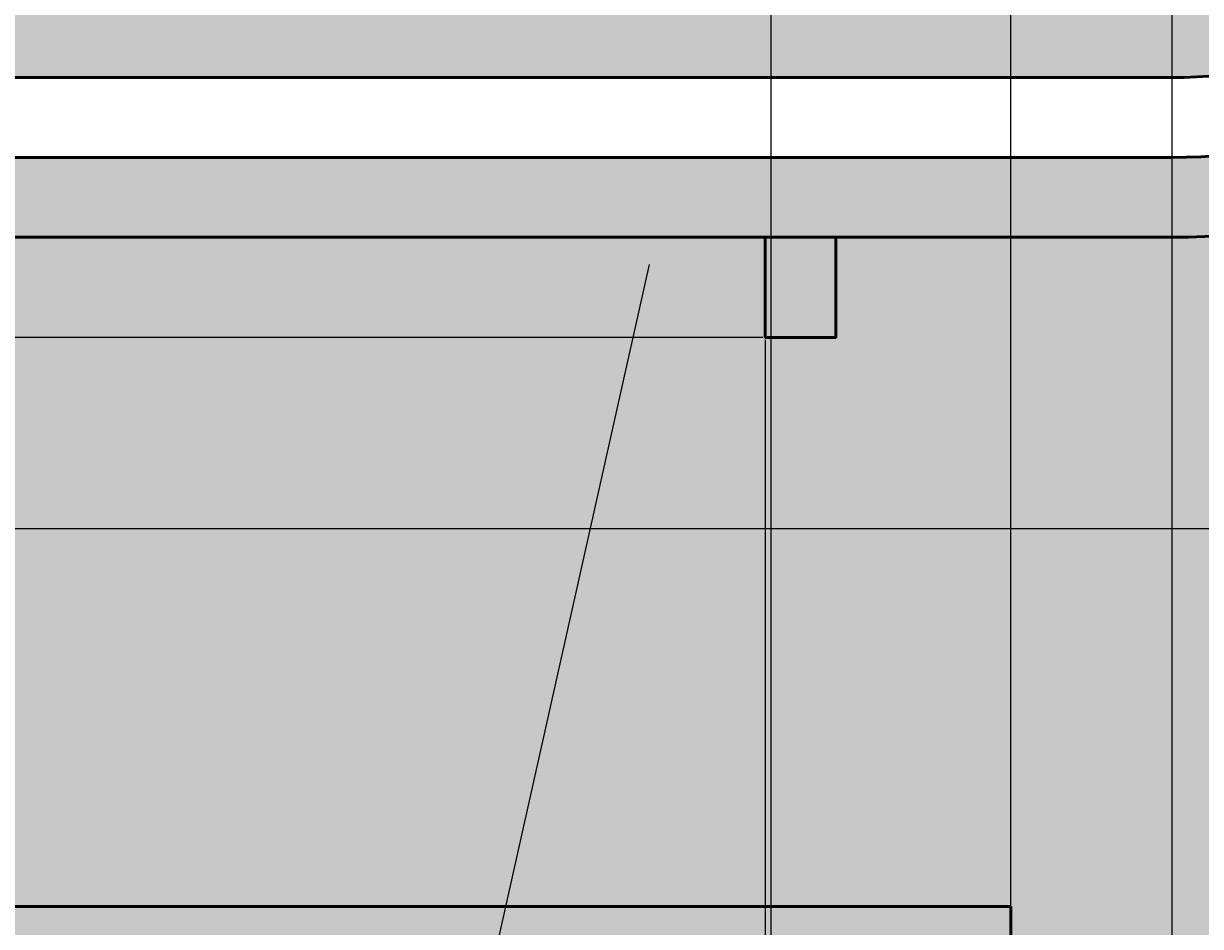
# Model space of a CAD drawing. Units: inches. Extents: x -12 to 334, y -10 to 186.
# Tile 50 of 77: x 198 to 227, y 46 to 69. Entities that reach past the tile are written whole.
import ezdxf
from ezdxf import colors
from ezdxf.entities.mleader import LeaderData, LeaderLine
from ezdxf.math import Vec2, Vec3

# ---------------------------------------------------------------- set-up
doc = ezdxf.new("R2010")
doc.units = ezdxf.units.IN
doc.header["$MEASUREMENT"] = 0
for name, color, linetype, lineweight in [('M-ANNO-TEXT', 3, 'Continuous', 25), ('M-DIMS', 2, 'Continuous', 18), ('M-EQPM', 7, 'Continuous', 50), ('M-EQPM-PATT', 8, 'Continuous', 18)]:
    doc.layers.add(name, color=color, linetype=linetype, lineweight=lineweight)
doc.styles.get("Standard").update_dxf_attribs({"font": 'arial.ttf'})
doc.dimstyles.get("Standard").update_dxf_attribs({"dimtxt": 0.18, "dimasz": 0.18, "dimexe": 0.18, "dimexo": 0.0625, "dimgap": 0.09, "dimtad": 0, "dimtih": 1, "dimtoh": 1, "dimdec": 4, "dimzin": 0, "dimdsep": 46, "dimtxsty": 'Standard', "dimcen": 0.09, "dimadec": 0, "dimazin": 0, "dimtfac": 1, "dimtdec": 4, "dimtofl": 0, "dimtmove": 0, "dimatfit": 3, "dimfxl": 1, "dimtolj": 1, "dimtzin": 0, "dimarcsym": 0})

# ---------------------------------------------------------------- blocks, each defined once
blk = doc.blocks.new('*D1')
at = {"layer": 'Defpoints', "color": 0, "transparency": 16777216}
for p in [(281.426, 91.899), (3.376, 80.692), (281.426, 14.304)]:
    blk.add_point(p, dxfattribs=at)
at = {"layer": 'M-DIMS', "color": 0, "lineweight": -2, "transparency": 16777216}
for p, q in [((281.426, 91.836), (281.426, 14.124)), ((3.376, 80.629), (3.376, 14.124)), ((3.556, 14.304), (141.935, 14.304)), ((281.246, 14.304), (142.867, 14.304))]:
    blk.add_line(p, q, dxfattribs=at)
at = {"layer": 'M-DIMS', "color": 0, "transparency": 16777216}
for points in [[(3.556, 14.334), (3.556, 14.274), (3.376, 14.304)], [(281.246, 14.334), (281.246, 14.274), (281.426, 14.304)]]:
    blk.add_solid(points, dxfattribs=at)
at = {"layer": 'M-DIMS', "color": 0, "transparency": 16777216, "insert": (142.401, 14.304), "char_height": 0.18, "attachment_point": 5}
blk.add_mtext('\\A1;278.05', dxfattribs=at)
blk = doc.blocks.new('*D17')
at = {"layer": 'Defpoints', "color": 0, "transparency": 16777216}
for p in [(106.177, 102.896), (105.892, 56.321), (295.976, 56.321)]:
    blk.add_point(p, dxfattribs=at)
at = {"layer": 'M-DIMS', "color": 0, "lineweight": -2, "transparency": 16777216}
for p, q in [((106.24, 102.896), (296.156, 102.896)), ((295.976, 102.716), (295.976, 79.79)), ((295.976, 56.501), (295.976, 79.426)), ((105.954, 56.321), (296.156, 56.321))]:
    blk.add_line(p, q, dxfattribs=at)
at = {"layer": 'M-DIMS', "color": 0, "transparency": 16777216}
for points in [[(295.946, 102.716), (296.006, 102.716), (295.976, 102.896)], [(295.946, 56.501), (296.006, 56.501), (295.976, 56.321)]]:
    blk.add_solid(points, dxfattribs=at)
at = {"layer": 'M-DIMS', "color": 0, "transparency": 16777216, "insert": (295.976, 79.608), "char_height": 0.18, "attachment_point": 5}
blk.add_mtext('\\A1;46.575', dxfattribs=at)
blk = doc.blocks.new('*D27')
at = {"layer": 'Defpoints', "color": 0, "transparency": 16777216}
for p in [(238.576, 169.385), (216.576, 32.854), (238.576, 32.854)]:
    blk.add_point(p, dxfattribs=at)
at = {"layer": 'M-DIMS', "color": 0, "lineweight": -2, "transparency": 16777216}
for p, q in [((216.576, 32.917), (216.576, 169.565)), ((238.576, 32.917), (238.576, 169.565)), ((216.756, 169.385), (227.357, 169.385)), ((238.396, 169.385), (227.796, 169.385))]:
    blk.add_line(p, q, dxfattribs=at)
at = {"layer": 'M-DIMS', "color": 0, "transparency": 16777216}
for points in [[(216.756, 169.415), (216.756, 169.355), (216.576, 169.385)], [(238.396, 169.415), (238.396, 169.355), (238.576, 169.385)]]:
    blk.add_solid(points, dxfattribs=at)
at = {"layer": 'M-DIMS', "color": 0, "transparency": 16777216, "insert": (227.576, 169.385), "char_height": 0.18, "attachment_point": 5}
blk.add_mtext('\\A1;22', dxfattribs=at)
blk = doc.blocks.new('*D28')
at = {"layer": 'Defpoints', "color": 0, "transparency": 16777216}
for p in [(232.576, 169.385), (222.576, 30.854), (232.576, 30.854)]:
    blk.add_point(p, dxfattribs=at)
at = {"layer": 'M-DIMS', "color": 0, "lineweight": -2, "transparency": 16777216}
for p, q in [((222.576, 30.917), (222.576, 169.565)), ((232.576, 30.917), (232.576, 169.565)), ((222.756, 169.385), (227.366, 169.385)), ((232.396, 169.385), (227.786, 169.385))]:
    blk.add_line(p, q, dxfattribs=at)
at = {"layer": 'M-DIMS', "color": 0, "transparency": 16777216}
for points in [[(222.756, 169.415), (222.756, 169.355), (222.576, 169.385)], [(232.396, 169.415), (232.396, 169.355), (232.576, 169.385)]]:
    blk.add_solid(points, dxfattribs=at)
at = {"layer": 'M-DIMS', "color": 0, "transparency": 16777216, "insert": (227.576, 169.385), "char_height": 0.18, "attachment_point": 5}
blk.add_mtext('\\A1;10', dxfattribs=at)
blk = doc.blocks.new('*D32')
at = {"layer": 'Defpoints', "color": 0, "transparency": 16777216}
for p in [(170.908, 61.105), (216.428, 61.105), (216.428, 14.304)]:
    blk.add_point(p, dxfattribs=at)
at = {"layer": 'M-DIMS', "color": 0, "lineweight": -2, "transparency": 16777216}
for p, q in [((170.908, 61.042), (170.908, 14.124)), ((216.428, 61.042), (216.428, 14.124)), ((171.088, 14.304), (193.271, 14.304)), ((216.248, 14.304), (194.064, 14.304))]:
    blk.add_line(p, q, dxfattribs=at)
at = {"layer": 'M-DIMS', "color": 0, "transparency": 16777216}
for points in [[(171.088, 14.334), (171.088, 14.274), (170.908, 14.304)], [(216.248, 14.334), (216.248, 14.274), (216.428, 14.304)]]:
    blk.add_solid(points, dxfattribs=at)
at = {"layer": 'M-DIMS', "color": 0, "transparency": 16777216, "insert": (193.668, 14.304), "char_height": 0.18, "attachment_point": 5}
blk.add_mtext('\\A1;45.52', dxfattribs=at)
blk = doc.blocks.new('*D33')
at = {"layer": 'Defpoints', "color": 0, "transparency": 16777216}
for p in [(226.608, 79.754), (216.428, 61.105), (226.608, 14.304)]:
    blk.add_point(p, dxfattribs=at)
at = {"layer": 'M-DIMS', "color": 0, "lineweight": -2, "transparency": 16777216}
for p, q in [((226.608, 79.692), (226.608, 14.124)), ((216.428, 61.042), (216.428, 14.124)), ((216.608, 14.304), (221.133, 14.304)), ((226.428, 14.304), (221.903, 14.304))]:
    blk.add_line(p, q, dxfattribs=at)
at = {"layer": 'M-DIMS', "color": 0, "transparency": 16777216}
for points in [[(216.608, 14.334), (216.608, 14.274), (216.428, 14.304)], [(226.428, 14.334), (226.428, 14.274), (226.608, 14.304)]]:
    blk.add_solid(points, dxfattribs=at)
at = {"layer": 'M-DIMS', "color": 0, "transparency": 16777216, "insert": (221.518, 14.304), "char_height": 0.18, "attachment_point": 5}
blk.add_mtext('\\A1;10.18', dxfattribs=at)
blk = doc.blocks.new('*D35')
at = {"layer": 'Defpoints', "color": 0, "transparency": 16777216}
for p in [(216.428, 98.108), (-11.174, 61.105), (216.428, 61.105)]:
    blk.add_point(p, dxfattribs=at)
at = {"layer": 'M-DIMS', "color": 0, "lineweight": -2, "transparency": 16777216}
for p, q in [((216.365, 98.108), (-11.354, 98.108)), ((-11.174, 97.928), (-11.174, 79.788)), ((-11.174, 61.285), (-11.174, 79.424)), ((216.365, 61.105), (-11.354, 61.105))]:
    blk.add_line(p, q, dxfattribs=at)
at = {"layer": 'M-DIMS', "color": 0, "transparency": 16777216}
for points in [[(-11.204, 97.928), (-11.144, 97.928), (-11.174, 98.108)], [(-11.204, 61.285), (-11.144, 61.285), (-11.174, 61.105)]]:
    blk.add_solid(points, dxfattribs=at)
at = {"layer": 'M-DIMS', "color": 0, "transparency": 16777216, "insert": (-11.174, 79.606), "char_height": 0.18, "attachment_point": 5}
blk.add_mtext('\\A1;37', dxfattribs=at)
blk = doc.blocks.new('*D39')
at = {"layer": 'Defpoints', "color": 0, "transparency": 16777216}
for p in [(279.726, 80.692), (-11.174, 45.854), (269.381, 45.854)]:
    blk.add_point(p, dxfattribs=at)
at = {"layer": 'M-DIMS', "color": 0, "lineweight": -2, "transparency": 16777216}
for p, q in [((279.664, 80.692), (-11.354, 80.692)), ((-11.174, 80.512), (-11.174, 63.455)), ((-11.174, 46.034), (-11.174, 63.091)), ((269.318, 45.854), (-11.354, 45.854))]:
    blk.add_line(p, q, dxfattribs=at)
at = {"layer": 'M-DIMS', "color": 0, "transparency": 16777216}
for points in [[(-11.204, 80.512), (-11.144, 80.512), (-11.174, 80.692)], [(-11.204, 46.034), (-11.144, 46.034), (-11.174, 45.854)]]:
    blk.add_solid(points, dxfattribs=at)
at = {"layer": 'M-DIMS', "color": 0, "transparency": 16777216, "insert": (-11.174, 63.273), "char_height": 0.18, "attachment_point": 5}
blk.add_mtext('\\A1;34.84', dxfattribs=at)
blk = doc.blocks.new('*D41')
at = {"layer": 'Defpoints', "color": 0, "transparency": 16777216}
for p in [(190.169, 91.899), (277.343, 68.515)]:
    blk.add_point(p, dxfattribs=at)
at = {"layer": 'M-DIMS', "color": 0, "lineweight": -2, "transparency": 16777216}
for p, q in [((190.169, 91.809), (190.169, 91.989)), ((190.079, 91.899), (190.259, 91.899)), ((329.648, 54.485), (277.517, 68.469)), ((329.828, 54.485), (329.648, 54.485))]:
    blk.add_line(p, q, dxfattribs=at)
at = {"layer": 'M-DIMS', "color": 0, "transparency": 16777216}
blk.add_solid([(277.525, 68.498), (277.509, 68.44), (277.343, 68.515)], dxfattribs=at)
at = {"layer": 'M-DIMS', "color": 0, "transparency": 16777216, "insert": (330.307, 54.485), "char_height": 0.18, "attachment_point": 5}
blk.add_mtext('\\A1;R90.26', dxfattribs=at)

msp = doc.modelspace()

# ---------------------------------------------------------------- hatches: boundary and pattern name
at = {"layer": 'M-EQPM-PATT'}
h = msp.add_hatch(color=256, dxfattribs=at)
h.set_gradient(color1=(99, 100, 102), color2=(99, 100, 102), tint=1)
h.paths.add_polyline_path([(4.3766, 80.754, -0.4132606), (23.5807, 99.8958), (37.1002, 99.8958), (37.1002, 127.7078), (32.1002, 127.7078), (32.1002, 125.2078), (36.1002, 125.2078), (36.1002, 100.8958), (23.5807, 100.8958, 1), (23.5807, 60.4872), (36.1002, 60.4872), (36.1002, 36.1752), (32.1002, 36.1752), (32.1002, 33.6752), (37.1002, 33.6752), (37.1002, 61.4872), (23.5807, 61.4872, -0.384914), (4.4744, 78.754), (72.9244, 78.754), (72.9244, 69.6117), (75.9244, 69.6117), (75.9244, 89.8963), (72.9244, 89.8963), (72.9244, 80.754)])
h.paths.add_polyline_path([(54.1002, 125.2078), (58.1002, 125.2078), (58.1002, 127.7078), (53.1002, 127.7078), (53.1002, 99.8958), (64.5, 99.8958), (64.5, 109.0583), (63.5, 109.0583), (63.5, 100.8958), (54.1002, 100.8958)], flags=17)
h.paths.add_polyline_path([(53.1002, 33.6752), (58.1002, 33.6752), (58.1002, 36.1752), (54.1002, 36.1752), (54.1002, 60.4872), (64.2068, 60.4872), (64.2068, 49.4497), (87.8879, 49.4497), (87.8879, 55.3205), (104.8919, 55.3205), (104.8919, 30.8541), (99.8919, 30.8541), (99.8919, 28.8541), (105.8919, 28.8541), (105.8919, 56.3205), (87.8879, 56.3205), (87.8879, 63.6117), (86.8879, 63.6117), (86.8879, 50.4497), (65.0061, 50.4497), (65.0061, 63.6117), (64.5, 63.6117), (64.5, 61.4872), (53.1002, 61.4872)])
h.paths.add_polyline_path([(121.8919, 28.8541), (121.8919, 30.8541), (116.8919, 30.8541), (116.8919, 45.8541), (209.6965, 45.8541), (209.9204, 46.8541), (115.8919, 46.8541), (115.8919, 28.8541)])
h.paths.add_polyline_path([(221.5761, 32.8541), (216.5761, 32.8541), (216.5761, 30.8541), (222.5761, 30.8541), (222.5761, 46.8541), (209.9204, 46.8541), (209.6965, 45.8541), (221.5761, 45.8541)])
h.paths.add_polyline_path([(233.5761, 45.8541), (249.8485, 45.8541), (249.3759, 46.8541), (232.5761, 46.8541), (232.5761, 30.8541), (238.5761, 30.8541), (238.5761, 32.8541), (233.5761, 32.8541)])
h = msp.add_hatch(color=256, dxfattribs=at)
h.set_gradient(color1=(205, 32, 39), color2=(205, 32, 39), tint=1)
h.paths.add_polyline_path([(64.5, 80.754), (64.5, 89.8963), (226.6083, 89.8963, -1), (226.6083, 69.6117), (64.5, 69.6117), (64.5, 78.754), (4.4744, 78.754, 0.384914), (23.5807, 61.4872), (37.1002, 61.4872), (37.1002, 33.6752), (53.1002, 33.6752), (53.1002, 61.4872), (64.5, 61.4872), (64.5, 63.6117), (226.6083, 63.6117, 1), (226.6083, 95.8963), (64.5, 95.8963), (64.5, 99.8958), (53.1002, 99.8958), (53.1002, 127.7078), (37.1002, 127.7078), (37.1002, 99.8958), (23.5807, 99.8958, 0.4132606), (4.3766, 80.754)])
h.paths.add_polyline_path([(64.5, 91.8963), (64.5, 93.8963), (226.6083, 93.8963, -1), (226.6083, 65.6117), (64.5, 65.6117), (64.5, 67.6117), (226.6083, 67.6117, 1), (226.6083, 91.8963)], flags=16)
h = msp.add_hatch(color=256, dxfattribs=at)
h.set_gradient(color1=(99, 100, 102), color2=(99, 100, 102), tint=1)
h.paths.add_polyline_path([(72.9244, 95.8963), (75.9244, 95.8963), (75.9244, 109.0583), (72.9244, 109.0583)])
h.paths.add_polyline_path([(72.9244, 50.4497), (75.9244, 50.4497), (75.9244, 63.6117), (72.9244, 63.6117)])
h.paths.add_polyline_path([(75.9244, 91.8963), (75.9244, 93.8963), (72.9244, 93.8963), (72.9244, 91.8963)])
h.paths.add_polyline_path([(75.9244, 65.6117), (75.9244, 67.6117), (72.9244, 67.6117), (72.9244, 65.6117)])
h.paths.add_polyline_path([(129.093, 69.6117), (130.8573, 69.6117), (130.8573, 89.8963), (129.093, 89.8963)])
h.paths.add_polyline_path([(129.093, 98.1081), (129.093, 95.8963), (130.8573, 95.8963), (130.8573, 98.1081)])
h.paths.add_polyline_path([(130.8573, 61.1045), (130.8573, 63.6117), (129.093, 63.6117), (129.093, 61.1045)])
h.paths.add_polyline_path([(170.9079, 69.6117), (172.6722, 69.6117), (172.6722, 89.8963), (170.9079, 89.8963)])
h.paths.add_polyline_path([(172.6722, 95.8963), (172.6722, 98.1081), (170.9079, 98.1081), (170.9079, 95.8963)])
h.paths.add_polyline_path([(170.9079, 61.1045), (172.6722, 61.1045), (172.6722, 63.6117), (170.9079, 63.6117)])
h.paths.add_polyline_path([(218.1922, 63.6117), (216.4278, 63.6117), (216.4278, 61.1045), (218.1922, 61.1045)])
h.paths.add_polyline_path([(216.4278, 69.6117), (218.1922, 69.6117), (218.1922, 89.8963), (216.4278, 89.8963)])
h.paths.add_polyline_path([(216.4278, 95.8963), (218.1922, 95.8963), (218.1922, 98.1081), (216.4278, 98.1081)])
h = msp.add_hatch(color=256, dxfattribs=at)
h.set_gradient(color1=(94, 103, 175), color2=(94, 103, 175), tint=1)
h.paths.add_polyline_path([(129.093, 89.8963), (86.8879, 89.8963), (86.8879, 69.6117), (129.093, 69.6117)], flags=17)
h.paths.add_polyline_path([(170.9079, 89.8963), (130.8573, 89.8963), (130.8573, 69.6117), (170.9079, 69.6117)], flags=17)
h.paths.add_polyline_path([(216.4278, 89.8963), (172.6722, 89.8963), (172.6722, 69.6117), (216.4278, 69.6117)], flags=17)
h.paths.add_polyline_path([(245.9354, 82.6969), (247.9354, 82.6969), (247.9354, 46.8541), (268.3808, 46.8541, 0.0998398), (279.7263, 80.6915), (251.9801, 80.6915, 0.4142136), (231.7758, 100.8958), (84.7229, 100.8958), (84.7229, 109.0583), (83.7229, 109.0583), (83.7229, 95.8963), (129.093, 95.8963), (129.093, 98.1081), (130.8573, 98.1081), (130.8573, 95.8963), (170.9079, 95.8963), (170.9079, 98.1081), (172.6722, 98.1081), (172.6722, 95.8963), (216.4278, 95.8963), (216.4278, 98.1081), (218.1922, 98.1081), (218.1922, 95.8963), (226.6083, 95.8963, -1), (226.6083, 63.6117), (218.1922, 63.6117), (218.1922, 61.1045), (216.4278, 61.1045), (216.4278, 63.6117), (172.6722, 63.6117), (172.6722, 61.1045), (170.9079, 61.1045), (170.9079, 63.6117), (130.8573, 63.6117), (130.8573, 61.1045), (129.093, 61.1045), (129.093, 63.6117), (87.8879, 63.6117), (87.8879, 56.3205), (105.8919, 56.3205), (105.8919, 28.8541), (115.8919, 28.8541), (115.8919, 46.8541), (222.5761, 46.8541), (222.5761, 30.8541), (232.5761, 30.8541), (232.5761, 46.8541), (245.9354, 46.8541)])
h.paths.add_polyline_path([(86.8879, 89.8963), (75.9244, 89.8963), (75.9244, 69.6117), (86.8879, 69.6117)])
h.paths.add_polyline_path([(83.7229, 109.0583), (75.9244, 109.0583), (75.9244, 95.8963), (83.7229, 95.8963)])
h.paths.add_polyline_path([(226.6083, 89.8963), (218.1922, 89.8963), (218.1922, 69.6117), (226.6083, 69.6117, 1)], flags=17)
h = msp.add_hatch(color=256, dxfattribs=at)
h.set_gradient(color1=(0, 0, 255), color2=(0, 0, 255), tint=1)
h.paths.add_polyline_path([(84.7229, 100.8958), (84.7229, 109.0583), (83.7229, 109.0583), (83.7229, 95.8963), (129.093, 95.8963), (129.093, 98.1081), (130.8573, 98.1081), (130.8573, 95.8963), (170.9079, 95.8963), (170.9079, 98.1081), (172.6722, 98.1081), (172.6722, 95.8963), (216.4278, 95.8963), (216.4278, 98.1081), (218.1922, 98.1081), (218.1922, 95.8963), (226.6083, 95.8963, -1), (226.6083, 63.6117), (218.1922, 63.6117), (218.1922, 61.1045), (216.4278, 61.1045), (216.4278, 63.6117), (172.6722, 63.6117), (172.6722, 61.1045), (170.9079, 61.1045), (170.9079, 63.6117), (130.8573, 63.6117), (130.8573, 61.1045), (129.093, 61.1045), (129.093, 63.6117), (87.8879, 63.6117), (87.8879, 56.3205), (105.8919, 56.3205), (105.8919, 28.8541), (115.8919, 28.8541), (115.8919, 46.8541), (222.5761, 46.8541), (222.5761, 30.8541), (232.5761, 30.8541), (232.5761, 46.8541), (245.9354, 46.8541), (245.9354, 82.6969), (247.9354, 82.6969), (247.9354, 46.8541), (268.3808, 46.8541, 0.0998398), (279.7263, 80.6915), (251.9801, 80.6915, 0.4142136), (231.7758, 100.8958)])

# ---------------------------------------------------------------- linework, layer by layer
at = {"layer": 'M-EQPM'}
for p, q in [((222.5761, 46.8541), (115.8919, 46.8541)), ((222.5761, 30.8541), (222.5761, 46.8541))]:
    msp.add_line(p, q, dxfattribs=at)
for points in [[(64.5, 63.6117), (226.6083, 63.6117, 1), (226.6083, 95.8963), (64.5, 95.8963)], [(64.5, 65.6117), (226.6083, 65.6117, 1), (226.6083, 93.8963), (64.5, 93.8963)], [(64.5, 67.6117), (226.6083, 67.6117, 1), (226.6083, 91.8963), (64.5, 91.8963)]]:
    msp.add_lwpolyline(points, format="xyb", dxfattribs=at)
msp.add_lwpolyline([(218.1922, 63.6117), (218.1922, 61.1045), (216.4278, 61.1045), (216.4278, 63.6117)], dxfattribs=at)

# ---------------------------------------------------------------- dimensions: what is measured, and where the dimension line sits
at = {"layer": 'M-DIMS'}
for base, p1, p2, override, picture, middle in [((238.5761, 169.3845), (216.5761, 32.8541), (238.5761, 32.8541), {"dimdec": 0, "dimlfac": 1, "dimrnd": 0, "dimzin": 0, "dimdsep": 46, "dimlunit": 2}, '*D27', (227.5761, 169.3845)), ((232.5761, 169.3845), (222.5761, 30.8541), (232.5761, 30.8541), {"dimdec": 0, "dimlfac": 1, "dimrnd": 0, "dimzin": 0, "dimdsep": 46, "dimlunit": 2}, '*D28', (227.5761, 169.3845)), ((281.4256, 14.3041), (3.3765, 80.6915), (281.4256, 91.8988), {"dimdec": 2, "dimlfac": 1, "dimrnd": 0, "dimzin": 0, "dimdsep": 46, "dimlunit": 2}, '*D1', (142.401, 14.3041)), ((226.6083, 14.3041), (216.4278, 61.1045), (226.6083, 79.754), {"dimdec": 2, "dimlfac": 1, "dimrnd": 0, "dimzin": 0, "dimdsep": 46, "dimlunit": 2}, '*D33', (221.5181, 14.3041)), ((216.4278, 14.3041), (170.9079, 61.1045), (216.4278, 61.1045), {"dimdec": 2, "dimlfac": 1, "dimrnd": 0, "dimzin": 0, "dimdsep": 46, "dimlunit": 2}, '*D32', (193.6678, 14.3041))]:
    dim = msp.add_linear_dim(base=base, p1=p1, p2=p2, dimstyle='Standard', override=override, dxfattribs=at)
    dim.commit()
    dim.dimension.update_dxf_attribs({"geometry": picture, "text_midpoint": middle})
for base, p1, p2, override, picture, middle in [((295.9756, 56.3205), (106.1771, 102.8958), (105.8919, 56.3205), {"dimdec": 3, "dimlfac": 1, "dimrnd": 0, "dimzin": 0, "dimdsep": 46, "dimlunit": 2}, '*D17', (295.9756, 79.6082)), ((-11.1736, 61.1045), (216.4278, 98.1081), (216.4278, 61.1045), {"dimdec": 0, "dimlfac": 1, "dimrnd": 0, "dimzin": 0, "dimdsep": 46, "dimlunit": 2}, '*D35', (-11.1735, 79.6063)), ((-11.1736, 45.8541), (279.7263, 80.6915), (269.3808, 45.8541), {"dimdec": 2, "dimlfac": 1, "dimrnd": 0, "dimzin": 0, "dimdsep": 46, "dimlunit": 2}, '*D39', (-11.1735, 63.2728))]:
    dim = msp.add_linear_dim(base=base, p1=p1, p2=p2, angle=90, dimstyle='Standard', override=override, dxfattribs=at)
    dim.commit()
    dim.dimension.update_dxf_attribs({"geometry": picture, "text_midpoint": middle})
dim = msp.add_radius_dim(center=(190.1689, 91.8988), mpoint=(277.3431, 68.5153), dimstyle='Standard', override={"dimdec": 2, "dimlfac": 1, "dimrnd": 0, "dimzin": 0, "dimdsep": 46, "dimlunit": 2}, dxfattribs=at)
dim.commit()
dim.dimension.update_dxf_attribs({"geometry": '*D41', "text_midpoint": (330.3074, 54.4851), "dimtype": 164})

# ---------------------------------------------------------------- leaders
at = {"layer": 'M-ANNO-TEXT'}
ml = msp.add_multileader_mtext('Standard', dxfattribs=at)
ml.set_content('u-tubes', color=256)
ml.set_leader_properties()
ml.build(insert=Vec2(0, 0))
ml.multileader.update_dxf_attribs({"dogleg_length": 0.36, "arrow_head_size": 0.7})
ctx = ml.context
ctx.base_point, ctx.arrow_head_size, ctx.landing_gap_size, ctx.plane_origin = Vec3(183.1578, 33.1882), 0.7, 0.09, Vec3(168.0474, 30.6523)
ctx.text_align_type = 2
notes = []
notes.append((ctx, [(1, (1, 1, 0), (206.8598, 33.1882), (-1, 0), 5.4565, [(0, [(213.6735, 63.6117)], 0, [])])]))
ctx.mtext.insert, ctx.mtext.alignment, ctx.mtext.flow_direction = Vec3(201.3133, 35.2209), 3, 5
for ctx, leaders in notes:
    for number, flags, end, landing, length, lines in leaders:
        leader = LeaderData()
        leader.index, (leader.has_last_leader_line, leader.has_dogleg_vector, leader.attachment_direction) = number, flags
        leader.last_leader_point, leader.dogleg_vector, leader.dogleg_length = Vec3(end), Vec3(landing), length
        for number, points, colour, breaks in lines:
            line = LeaderLine()
            line.index, line.vertices, line.color, line.breaks = number, Vec3.list(points), colors.encode_raw_color(colour), breaks
            leader.lines.append(line)
        ctx.leaders.append(leader)

doc.saveas('drawing.dxf')
